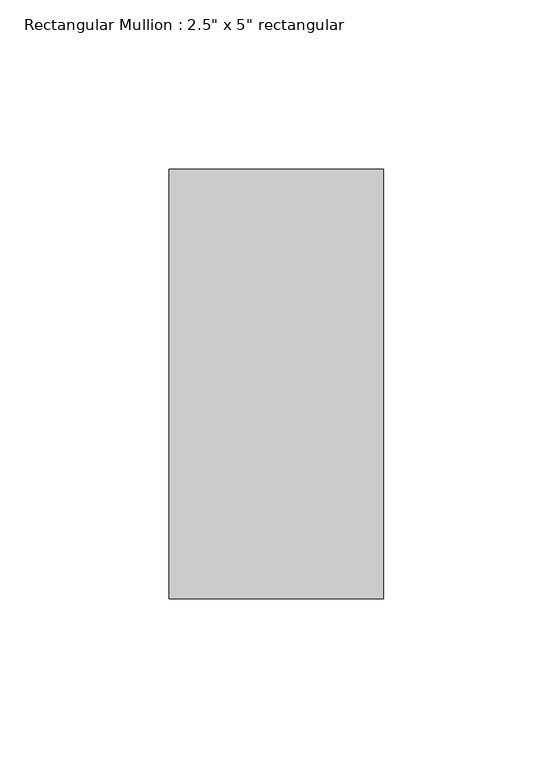
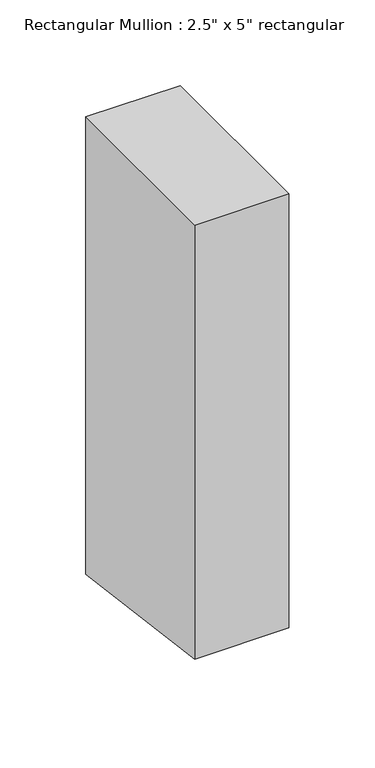
"""IFC4 building model written with IfcOpenShell, lengths in millimetres: member geometry."""

from ifc_helpers import new_model, si_unit, frame, origin, place, context, project, spatial, polyline, outline, extrude, source, transform, mapped, element, save


def member_068c4367(model_context):
    return source(origin(), model_context, "Body", "SweptSolid", [
        extrude(outline(polyline([(-63.5, 0.0), (63.5, 0.0), (63.5, -325.3541629), (-63.5, -308.8871146), (-63.5, 0.0)])), frame((-63.5, 0.0, 0.0), z_axis=(1.0, 0.0, 0.0), x_axis=(0.0, 1.0, 0.0)), (0.0, 0.0, 1.0), 63.5),
    ])


if __name__ == "__main__":
    model = new_model("IFC4")
    model_context = context("Model", 3, world=origin())
    ifc_project = project(units=[si_unit("LENGTHUNIT", "METRE", prefix="MILLI")], contexts=[model_context])
    site = spatial("IfcSite", under=ifc_project)
    building = spatial("IfcBuilding", under=site)
    placement = place(None, origin())
    member_shape = member_068c4367(model_context)
    element("IfcMember", 1, ObjectType="Rectangular Mullion : 2.5\" x 5\" rectangular", at=placement, inside=building, context=model_context, shape_type="MappedRepresentation", body=[
        mapped(member_shape, transform((0.0, 0.0, 0.0), x_axis=(1.0, 0.0, 0.0), y_axis=(0.0, 1.0, 0.0), z_axis=(0.0, 0.0, 1.0))),
    ])
    save(model, "model.ifc")

# Revit data of these elements
# Type "Rectangular Mullion : 2.5\" x 5\" rectangular"
#   built-in parameter 1007304 = 0.416667 (stored number, unit not read)
#   built-in parameter 1007301 = 0.104167 (stored number, unit not read)
#   built-in parameter 1007300 = 0.104167 (stored number, unit not read)
# Element 1 (IfcMember, "Rectangular Mullion : 2.5\" x 5\" rectangular")
#   Materials on its faces: "Iron, Ductile"
# Materials
#   "Iron, Ductile": class "Metal", colour RGB 0 0 0, transparency 0, Description = "Ductile cast iron", Cost = 0
